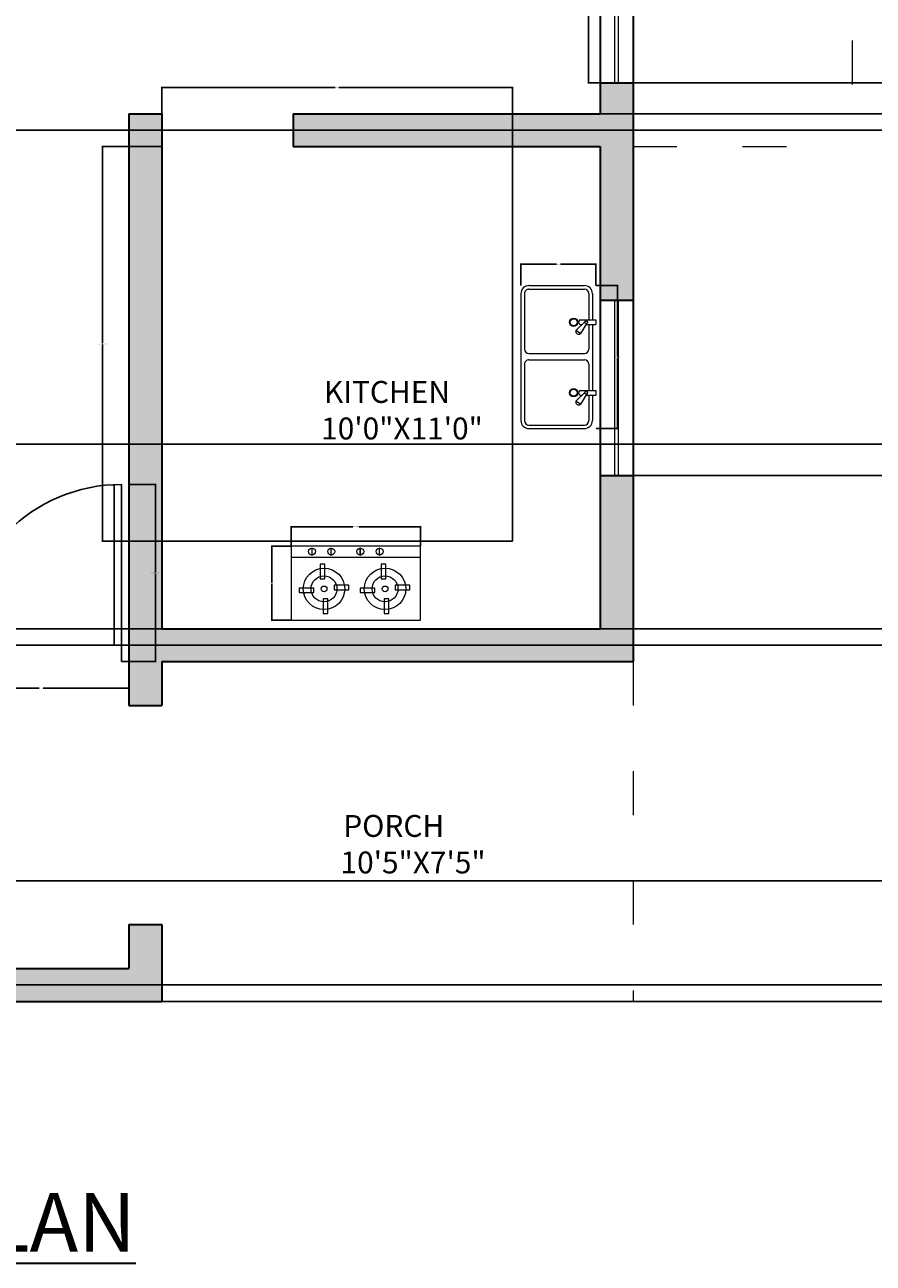
# Model space of a CAD drawing. Units: inches. Extents: x 5716 to 6907, y 12769 to 13594.
# Tile 2 of 17: x 6022 to 6254, y 12769 to 13109. Entities that reach past the tile are written whole.
import ezdxf

# ---------------------------------------------------------------- set-up
doc = ezdxf.new("R2010")
doc.units = ezdxf.units.IN
doc.linetypes.add('ACAD_ISO03W100', pattern=[30, 12, -18])
for name, color, linetype, lineweight in [('A-ANNO-DIMS', 2, 'Continuous', 18), ('A-ANNO-TEXT', 7, 'Continuous', 30), ('A-AREA-IDEN', 7, 'Continuous', 18), ('A-DOOR', 4, 'Continuous', 25), ('A-EQPM', 8, 'Continuous', 18), ('A-FLOR-CASE', 7, 'Continuous', 25), ('A-FLOR-FIXT', 9, 'Continuous', 18), ('A-FLOR-OVHD', 8, 'ACAD_ISO03W100', 18), ('A-GLAZ', 4, 'Continuous', 18), ('A-WALL', 7, 'Continuous', 35), ('A-WALL-PATT', 252, 'Continuous', 13)]:
    doc.layers.add(name, color=color, linetype=linetype, lineweight=lineweight)
doc.styles.get("Standard").update_dxf_attribs({"font": 'arial.ttf'})
doc.dimstyles.get("Standard").update_dxf_attribs({"dimtxt": 0.18, "dimasz": 0.18, "dimexe": 0.18, "dimexo": 0.0625, "dimgap": 0.09, "dimtad": 0, "dimtih": 1, "dimtoh": 1, "dimdec": 4, "dimzin": 0, "dimdsep": 46, "dimtxsty": 'Standard', "dimcen": 0.09, "dimadec": 0, "dimazin": 0, "dimtfac": 1, "dimtdec": 4, "dimtofl": 0, "dimtmove": 0, "dimatfit": 3, "dimfxl": 1, "dimtolj": 1, "dimtzin": 0, "dimarcsym": 0})

# ---------------------------------------------------------------- blocks, each defined once
blk = doc.blocks.new('A$C233D5AEA')
at = {"ltscale": 1000}
for p, q in [((375, 800), (65, 800)), ((375, 780), (65, 780)), ((20, 613.1), (20, 755)), ((40, 613.1), (40, 755)), ((400, 440), (400, 755)), ((420, 45), (420, 755)), ((51.1, 606.3), (87.4, 663.6)), ((111.9, 647), (62.8, 597.6)), ((87.4, 663.6), (111.9, 647)), ((55.4, 613.1), (0, 613.1)), ((0, 586.1), (0, 613.1)), ((88.6, 586.1), (0, 586.1)), ((20, 217.6), (20, 586.1)), ((40, 440), (40, 586.1)), ((87.8, 613.1), (78.2, 613.1)), ((40, 217.6), (40, 355)), ((375, 415), (65, 415)), ((375, 380), (65, 380)), ((400, 45), (400, 355)), ((55.4, 217.6), (0, 217.6)), ((0, 190.6), (0, 217.6)), ((51.1, 210.7), (87.4, 268)), ((111.9, 251.5), (62.8, 202)), ((87.8, 217.6), (78.2, 217.6)), ((87.4, 268), (111.9, 251.5)), ((88.6, 190.6), (0, 190.6)), ((20, 45), (20, 190.6)), ((40, 45), (40, 190.6)), ((375, 20), (65, 20)), ((375, 0), (65, 0))]:
    blk.add_line(p, q, dxfattribs=at)
for centre, radius in [((55.3, 599.7), 7.79), ((124.6, 599.4), 23.1), ((124.5, 599.4), 19.5), ((55.3, 204.2), 7.79), ((124.6, 204.7), 23.1), ((124.5, 204.7), 19.5)]:
    blk.add_circle(centre, radius, dxfattribs=at)
for centre, radius, start, end in [((65, 755), 45, 90, 180), ((65, 755), 25, 90, 180), ((375, 755), 45, 0, 90), ((375, 755), 25, 0, 90), ((97.5, 652.1), 15.3, 340.46224, 131.65496), ((82, 599.4), 14.9, 296.62368, 67.07956), ((65, 440), 25, 180, 270), ((375, 440), 25, 270, 0), ((65, 355), 25, 90, 180), ((375, 355), 25, 0, 90), ((97.5, 256.6), 15.3, 340.46913, 131.64807), ((82, 203.8), 14.9, 296.62368, 67.07956), ((65, 45), 45, 180, 270), ((65, 45), 25, 180, 270), ((375, 45), 45, 270, 0), ((375, 45), 25, 270, 0)]:
    blk.add_arc(centre, radius, start, end, dxfattribs=at)
blk = doc.blocks.new('A$C3BE07067')
at = {"rotation": 270}
blk.add_blockref('A$C233D5AEA', (0, 420), dxfattribs=at)
blk = doc.blocks.new('A$C67D72025')
at = {"ltscale": 1000}
for p, q in [((385.7, 234.1), (385.7, 209.4)), ((464.6, 234.1), (385.7, 234.1)), ((385.7, 209.4), (464.6, 209.4)), ((464.6, 209.4), (464.6, 234.1)), ((694.4, 59.5), (0, 59.5))]:
    blk.add_line(p, q, dxfattribs=at)
for points in [[(694.4, 396.8), (0, 396.8), (0, 0), (694.4, 0)], [(195.5, 283.6), (195.5, 362.4), (170.8, 362.4), (170.8, 283.6)], [(523.4, 283.6), (523.4, 362.4), (498.6, 362.4), (498.6, 283.6)], [(136.8, 234.1), (57.9, 234.1), (57.9, 209.4), (136.8, 209.4)], [(245, 224.8), (323.9, 224.8), (323.9, 249.5), (245, 249.5)], [(572.8, 224.8), (651.7, 224.8), (651.7, 249.5), (572.8, 249.5)], [(186.3, 175.3), (186.3, 96.5), (211, 96.5), (211, 175.3)], [(514.1, 175.3), (514.1, 96.5), (538.8, 96.5), (538.8, 175.3)], [(223.3, 47.3), (220, 47.3), (220, 9.9), (223.3, 9.9)], [(325.5, 47.3), (322.2, 47.3), (322.2, 9.9), (325.5, 9.9)], [(482.8, 47.3), (479.5, 47.3), (479.5, 9.9), (482.8, 9.9)], [(585, 47.3), (581.6, 47.3), (581.6, 9.9), (585, 9.9)]]:
    blk.add_lwpolyline(points, close=True, dxfattribs=at)
for centre, radius in [((190.9, 229.4), 111.3), ((518.7, 229.4), 111.3), ((190.9, 229.4), 69.6), ((518.7, 229.4), 69.6), ((190.9, 229.4), 15.5), ((518.7, 229.4), 15.5), ((220.3, 28.6), 18.6), ((323.9, 28.6), 18.6), ((480.1, 28.6), 18.6), ((583.7, 28.6), 18.6)]:
    blk.add_circle(centre, radius, dxfattribs=at)
blk = doc.blocks.new('DOOR-SWING-48IN')
for p, q in [((-2, 43.95), (-2, 0)), ((0, 44), (0, 0)), ((-46, 0), (-44, 0)), ((-44, 0), (-44, -4.5)), ((0, 0), (-2, 0)), ((2, 0), (0, 0)), ((0, 0), (0, -4.5)), ((-44, -4.5), (-46, -4.5)), ((0, -4.5), (2, -4.5))]:
    blk.add_line(p, q)
blk.add_arc((0, 0), 44, 90, 180)
blk = doc.blocks.new('WIN-GLAZING-48IN')
for p, q in [((0, 0), (0, 48)), ((1, 0), (1, 48))]:
    blk.add_line(p, q)
blk = doc.blocks.new('COUNTER-L-KITCHEN')
for p in [(0, 108), (-96, 0)]:
    blk.add_line(p, (0, 0))
blk = doc.blocks.new('*D31')
at = {"layer": 'A-ANNO-DIMS', "color": 0, "lineweight": -2, "transparency": 16777216}
for p, q in [((6182.96, 13140.65), (6175.64, 13140.65)), ((6175.82, 13140.47), (6175.82, 13116.83)), ((6175.82, 13092.83), (6175.82, 13116.47)), ((6182.96, 13092.65), (6175.64, 13092.65))]:
    blk.add_line(p, q, dxfattribs=at)
at = {"layer": 'A-ANNO-DIMS', "color": 0, "transparency": 16777216}
for points in [[(6175.79, 13140.47), (6175.85, 13140.47), (6175.82, 13140.65)], [(6175.79, 13092.83), (6175.85, 13092.83), (6175.82, 13092.65)]]:
    blk.add_solid(points, dxfattribs=at)
at = {"layer": 'Defpoints', "color": 0, "transparency": 16777216}
for p in [(6175.82, 13140.65), (6183.02, 13140.65), (6183.02, 13092.65)]:
    blk.add_point(p, dxfattribs=at)
at = {"layer": 'A-ANNO-DIMS', "color": 0, "transparency": 16777216, "insert": (6175.82, 13116.65), "char_height": 0.18, "attachment_point": 5}
blk.add_mtext('\\A1;WINDOW 48 TYP.', dxfattribs=at)
blk = doc.blocks.new('*D35')
at = {"layer": 'A-ANNO-DIMS', "color": 0, "lineweight": -2, "transparency": 16777216}
for p, q in [((6177.95, 13037.09), (6183.94, 13037.09)), ((6183.76, 13036.91), (6183.76, 13017.7)), ((6183.76, 12998.12), (6183.76, 13017.33)), ((6177.95, 12997.94), (6183.94, 12997.94))]:
    blk.add_line(p, q, dxfattribs=at)
at = {"layer": 'A-ANNO-DIMS', "color": 0, "transparency": 16777216}
for points in [[(6183.73, 13036.91), (6183.79, 13036.91), (6183.76, 13037.09)], [(6183.73, 12998.12), (6183.79, 12998.12), (6183.76, 12997.94)]]:
    blk.add_solid(points, dxfattribs=at)
at = {"layer": 'Defpoints', "color": 0, "transparency": 16777216}
for p in [(6177.88, 13037.09), (6177.88, 12997.94), (6183.76, 12997.94)]:
    blk.add_point(p, dxfattribs=at)
at = {"layer": 'A-ANNO-DIMS', "color": 0, "transparency": 16777216, "insert": (6183.76, 13017.51), "char_height": 0.18, "attachment_point": 5}
blk.add_mtext('\\A1;SINK 39 TYP.', dxfattribs=at)
blk = doc.blocks.new('*D36')
at = {"layer": 'A-ANNO-DIMS', "color": 0, "lineweight": -2, "transparency": 16777216}
for p, q in [((6157.33, 13037.15), (6157.33, 13043.14)), ((6157.51, 13042.96), (6167.08, 13042.96)), ((6177.7, 13042.96), (6168.14, 13042.96)), ((6177.88, 13037.15), (6177.88, 13043.14))]:
    blk.add_line(p, q, dxfattribs=at)
at = {"layer": 'A-ANNO-DIMS', "color": 0, "transparency": 16777216}
for points in [[(6157.51, 13042.99), (6157.51, 13042.93), (6157.33, 13042.96)], [(6177.7, 13042.99), (6177.7, 13042.93), (6177.88, 13042.96)]]:
    blk.add_solid(points, dxfattribs=at)
at = {"layer": 'Defpoints', "color": 0, "transparency": 16777216}
for p in [(6177.88, 13042.96), (6157.33, 13037.09), (6177.88, 13037.09)]:
    blk.add_point(p, dxfattribs=at)
at = {"layer": 'A-ANNO-DIMS', "color": 0, "transparency": 16777216, "insert": (6167.61, 13042.96), "char_height": 0.18, "attachment_point": 5}
blk.add_mtext('\\A1;21 TYP.', dxfattribs=at)
blk = doc.blocks.new('*D39')
at = {"layer": 'A-ANNO-DIMS', "color": 0, "lineweight": -2, "transparency": 16777216}
for p, q in [((6094.5, 12965.82), (6094.5, 12971.24)), ((6094.68, 12971.06), (6111.36, 12971.06)), ((6129.7, 12971.06), (6113.02, 12971.06)), ((6129.88, 12965.82), (6129.88, 12971.24))]:
    blk.add_line(p, q, dxfattribs=at)
at = {"layer": 'A-ANNO-DIMS', "color": 0, "transparency": 16777216}
for points in [[(6094.68, 12971.09), (6094.68, 12971.03), (6094.5, 12971.06)], [(6129.7, 12971.09), (6129.7, 12971.03), (6129.88, 12971.06)]]:
    blk.add_solid(points, dxfattribs=at)
at = {"layer": 'Defpoints', "color": 0, "transparency": 16777216}
for p in [(6094.5, 12971.06), (6094.5, 12965.75), (6129.88, 12965.75)]:
    blk.add_point(p, dxfattribs=at)
at = {"layer": 'A-ANNO-DIMS', "color": 0, "transparency": 16777216, "insert": (6112.19, 12971.06), "char_height": 0.18, "attachment_point": 5}
blk.add_mtext('\\A1;HOB 35 TYP.', dxfattribs=at)
blk = doc.blocks.new('*D40')
at = {"layer": 'A-ANNO-DIMS', "color": 0, "lineweight": -2, "transparency": 16777216}
for p, q in [((6094.44, 12965.75), (6089.02, 12965.75)), ((6089.2, 12965.57), (6089.2, 12955.83)), ((6089.2, 12945.72), (6089.2, 12955.46)), ((6094.44, 12945.54), (6089.02, 12945.54))]:
    blk.add_line(p, q, dxfattribs=at)
at = {"layer": 'A-ANNO-DIMS', "color": 0, "transparency": 16777216}
for points in [[(6089.17, 12965.57), (6089.23, 12965.57), (6089.2, 12965.75)], [(6089.17, 12945.72), (6089.23, 12945.72), (6089.2, 12945.54)]]:
    blk.add_solid(points, dxfattribs=at)
at = {"layer": 'Defpoints', "color": 0, "transparency": 16777216}
for p in [(6094.5, 12965.75), (6089.2, 12945.54), (6094.5, 12945.54)]:
    blk.add_point(p, dxfattribs=at)
at = {"layer": 'A-ANNO-DIMS', "color": 0, "transparency": 16777216, "insert": (6089.2, 12955.64), "char_height": 0.18, "attachment_point": 5}
blk.add_mtext('\\A1;20 TYP.', dxfattribs=at)
blk = doc.blocks.new('*D41')
at = {"layer": 'A-ANNO-DIMS', "color": 0, "lineweight": -2, "transparency": 16777216}
for p, q in [((6050.09, 12982.65), (6057.48, 12982.65)), ((6057.3, 12982.47), (6057.3, 12958.58)), ((6057.3, 12934.33), (6057.3, 12958.22)), ((6050.09, 12934.15), (6057.48, 12934.15))]:
    blk.add_line(p, q, dxfattribs=at)
at = {"layer": 'A-ANNO-DIMS', "color": 0, "transparency": 16777216}
for points in [[(6057.27, 12982.47), (6057.33, 12982.47), (6057.3, 12982.65)], [(6057.27, 12934.33), (6057.33, 12934.33), (6057.3, 12934.15)]]:
    blk.add_solid(points, dxfattribs=at)
at = {"layer": 'Defpoints', "color": 0, "transparency": 16777216}
for p in [(6050.02, 12982.65), (6057.3, 12982.65), (6050.02, 12934.15)]:
    blk.add_point(p, dxfattribs=at)
at = {"layer": 'A-ANNO-DIMS', "color": 0, "transparency": 16777216, "insert": (6057.3, 12958.4), "char_height": 0.18, "attachment_point": 5}
blk.add_mtext('\\A1;ENTRY DOOR 49 TYP.', dxfattribs=at)
blk = doc.blocks.new('*D42')
at = {"layer": 'A-ANNO-DIMS', "color": 0, "lineweight": -2, "transparency": 16777216}
for p, q in [((6002.02, 12934.09), (6002.02, 12926.69)), ((6050.02, 12934.09), (6050.02, 12926.69)), ((6002.2, 12926.87), (6025.49, 12926.87)), ((6049.84, 12926.87), (6026.55, 12926.87))]:
    blk.add_line(p, q, dxfattribs=at)
at = {"layer": 'A-ANNO-DIMS', "color": 0, "transparency": 16777216}
for points in [[(6002.2, 12926.9), (6002.2, 12926.84), (6002.02, 12926.87)], [(6049.84, 12926.9), (6049.84, 12926.84), (6050.02, 12926.87)]]:
    blk.add_solid(points, dxfattribs=at)
at = {"layer": 'Defpoints', "color": 0, "transparency": 16777216}
for p in [(6002.02, 12934.15), (6050.02, 12934.15), (6050.02, 12926.87)]:
    blk.add_point(p, dxfattribs=at)
at = {"layer": 'A-ANNO-DIMS', "color": 0, "transparency": 16777216, "insert": (6026.02, 12926.87), "char_height": 0.18, "attachment_point": 5}
blk.add_mtext('\\A1;48 TYP.', dxfattribs=at)
blk = doc.blocks.new('*D47')
at = {"layer": 'A-ANNO-DIMS', "color": 0, "lineweight": -2, "transparency": 16777216}
for p, q in [((6058.96, 13075.15), (6042.64, 13075.15)), ((6042.82, 13074.97), (6042.82, 13021.33)), ((6042.82, 12967.33), (6042.82, 13020.97)), ((6058.96, 12967.15), (6042.64, 12967.15))]:
    blk.add_line(p, q, dxfattribs=at)
at = {"layer": 'A-ANNO-DIMS', "color": 0, "transparency": 16777216}
for points in [[(6042.79, 13074.97), (6042.85, 13074.97), (6042.82, 13075.15)], [(6042.79, 12967.33), (6042.85, 12967.33), (6042.82, 12967.15)]]:
    blk.add_solid(points, dxfattribs=at)
at = {"layer": 'Defpoints', "color": 0, "transparency": 16777216}
for p in [(6042.82, 13075.15), (6059.02, 13075.15), (6059.02, 12967.15)]:
    blk.add_point(p, dxfattribs=at)
at = {"layer": 'A-ANNO-DIMS', "color": 0, "transparency": 16777216, "insert": (6042.82, 13021.15), "char_height": 0.18, "attachment_point": 5}
blk.add_mtext('\\A1;L-COUNTER 108 TYP.', dxfattribs=at)
blk = doc.blocks.new('*D48')
at = {"layer": 'A-ANNO-DIMS', "color": 0, "lineweight": -2, "transparency": 16777216}
for p, q in [((6059.02, 13075.21), (6059.02, 13091.53)), ((6059.2, 13091.35), (6106.49, 13091.35)), ((6154.84, 13091.35), (6107.55, 13091.35)), ((6155.02, 13075.21), (6155.02, 13091.53))]:
    blk.add_line(p, q, dxfattribs=at)
at = {"layer": 'A-ANNO-DIMS', "color": 0, "transparency": 16777216}
for points in [[(6059.2, 13091.38), (6059.2, 13091.32), (6059.02, 13091.35)], [(6154.84, 13091.38), (6154.84, 13091.32), (6155.02, 13091.35)]]:
    blk.add_solid(points, dxfattribs=at)
at = {"layer": 'Defpoints', "color": 0, "transparency": 16777216}
for p in [(6155.02, 13091.35), (6059.02, 13075.15), (6155.02, 13075.15)]:
    blk.add_point(p, dxfattribs=at)
at = {"layer": 'A-ANNO-DIMS', "color": 0, "transparency": 16777216, "insert": (6107.02, 13091.35), "char_height": 0.18, "attachment_point": 5}
blk.add_mtext('\\A1;96 TYP.', dxfattribs=at)
blk = doc.blocks.new('*D52')
at = {"layer": 'A-ANNO-DIMS', "color": 0, "lineweight": -2, "transparency": 16777216}
for p, q in [((6267.34, 13440.15), (5716.04, 13440.15)), ((5716.22, 13439.97), (5716.22, 13140.83)), ((5716.22, 12841.33), (5716.22, 13140.47)), ((6267.34, 12841.15), (5716.04, 12841.15))]:
    blk.add_line(p, q, dxfattribs=at)
at = {"layer": 'A-ANNO-DIMS', "color": 0, "transparency": 16777216}
for points in [[(5716.19, 13439.97), (5716.25, 13439.97), (5716.22, 13440.15)], [(5716.19, 12841.33), (5716.25, 12841.33), (5716.22, 12841.15)]]:
    blk.add_solid(points, dxfattribs=at)
at = {"layer": 'Defpoints', "color": 0, "transparency": 16777216}
for p in [(6267.41, 13440.15), (5716.22, 12841.15), (6267.41, 12841.15)]:
    blk.add_point(p, dxfattribs=at)
at = {"layer": 'A-ANNO-DIMS', "color": 0, "transparency": 16777216, "insert": (5716.22, 13140.65), "char_height": 0.18, "attachment_point": 5}
blk.add_mtext('\\A1;599', dxfattribs=at)
blk = doc.blocks.new('*D62')
at = {"layer": 'A-ANNO-DIMS', "color": 0, "lineweight": -2, "transparency": 16777216}
for p, q in [((6736.67, 13120.65), (5716.04, 13120.65)), ((5716.22, 13120.47), (5716.22, 13100.33)), ((5716.22, 13079.83), (5716.22, 13099.97)), ((6736.67, 13079.65), (5716.04, 13079.65))]:
    blk.add_line(p, q, dxfattribs=at)
at = {"layer": 'A-ANNO-DIMS', "color": 0, "transparency": 16777216}
for points in [[(5716.19, 13120.47), (5716.25, 13120.47), (5716.22, 13120.65)], [(5716.19, 13079.83), (5716.25, 13079.83), (5716.22, 13079.65)]]:
    blk.add_solid(points, dxfattribs=at)
at = {"layer": 'Defpoints', "color": 0, "transparency": 16777216}
for p in [(6736.73, 13120.65), (5716.22, 13079.65), (6736.73, 13079.65)]:
    blk.add_point(p, dxfattribs=at)
at = {"layer": 'A-ANNO-DIMS', "color": 0, "transparency": 16777216, "insert": (5716.22, 13100.15), "char_height": 0.18, "attachment_point": 5}
blk.add_mtext('\\A1;41', dxfattribs=at)
blk = doc.blocks.new('*D63')
at = {"layer": 'A-ANNO-DIMS', "color": 0, "lineweight": -2, "transparency": 16777216}
for p, q in [((6736.67, 13079.65), (5716.04, 13079.65)), ((5716.22, 13079.47), (5716.22, 13009.33)), ((5716.22, 12938.83), (5716.22, 13008.97)), ((6736.67, 12938.65), (5716.04, 12938.65))]:
    blk.add_line(p, q, dxfattribs=at)
at = {"layer": 'A-ANNO-DIMS', "color": 0, "transparency": 16777216}
for points in [[(5716.19, 13079.47), (5716.25, 13079.47), (5716.22, 13079.65)], [(5716.19, 12938.83), (5716.25, 12938.83), (5716.22, 12938.65)]]:
    blk.add_solid(points, dxfattribs=at)
at = {"layer": 'Defpoints', "color": 0, "transparency": 16777216}
for p in [(6736.73, 13079.65), (5716.22, 12938.65), (6736.73, 12938.65)]:
    blk.add_point(p, dxfattribs=at)
at = {"layer": 'A-ANNO-DIMS', "color": 0, "transparency": 16777216, "insert": (5716.22, 13009.15), "char_height": 0.18, "attachment_point": 5}
blk.add_mtext('\\A1;141', dxfattribs=at)
blk = doc.blocks.new('*D64')
at = {"layer": 'A-ANNO-DIMS', "color": 0, "lineweight": -2, "transparency": 16777216}
for p, q in [((6736.67, 12938.65), (5716.04, 12938.65)), ((5716.22, 12938.47), (5716.22, 12892.33)), ((5716.22, 12845.83), (5716.22, 12891.97)), ((6736.67, 12845.65), (5716.04, 12845.65))]:
    blk.add_line(p, q, dxfattribs=at)
at = {"layer": 'A-ANNO-DIMS', "color": 0, "transparency": 16777216}
for points in [[(5716.19, 12938.47), (5716.25, 12938.47), (5716.22, 12938.65)], [(5716.19, 12845.83), (5716.25, 12845.83), (5716.22, 12845.65)]]:
    blk.add_solid(points, dxfattribs=at)
at = {"layer": 'Defpoints', "color": 0, "transparency": 16777216}
for p in [(6736.73, 12938.65), (5716.22, 12845.65), (6736.73, 12845.65)]:
    blk.add_point(p, dxfattribs=at)
at = {"layer": 'A-ANNO-DIMS', "color": 0, "transparency": 16777216, "insert": (5716.22, 12892.15), "char_height": 0.18, "attachment_point": 5}
blk.add_mtext('\\A1;93', dxfattribs=at)
blk = doc.blocks.new('*D67')
at = {"layer": 'A-ANNO-DIMS', "color": 0, "lineweight": -2, "transparency": 16777216}
for p, q in [((5819.09, 12874.15), (6907.26, 12874.15)), ((6907.08, 12873.97), (6907.08, 12857.83)), ((6907.08, 12841.33), (6907.08, 12857.47)), ((5819.09, 12841.15), (6907.26, 12841.15))]:
    blk.add_line(p, q, dxfattribs=at)
at = {"layer": 'A-ANNO-DIMS', "color": 0, "transparency": 16777216}
for points in [[(6907.05, 12873.97), (6907.11, 12873.97), (6907.08, 12874.15)], [(6907.05, 12841.33), (6907.11, 12841.33), (6907.08, 12841.15)]]:
    blk.add_solid(points, dxfattribs=at)
at = {"layer": 'Defpoints', "color": 0, "transparency": 16777216}
for p in [(5819.02, 12874.15), (6907.08, 12874.15), (5819.02, 12841.15)]:
    blk.add_point(p, dxfattribs=at)
at = {"layer": 'A-ANNO-DIMS', "color": 0, "transparency": 16777216, "insert": (6907.08, 12857.65), "char_height": 0.18, "attachment_point": 5}
blk.add_mtext('\\A1;33', dxfattribs=at)
blk = doc.blocks.new('*D68')
at = {"layer": 'A-ANNO-DIMS', "color": 0, "lineweight": -2, "transparency": 16777216}
for p, q in [((5828.09, 12993.65), (6907.26, 12993.65)), ((6907.08, 12993.47), (6907.08, 12968.58)), ((6907.08, 12943.33), (6907.08, 12968.22)), ((5828.09, 12943.15), (6907.26, 12943.15))]:
    blk.add_line(p, q, dxfattribs=at)
at = {"layer": 'A-ANNO-DIMS', "color": 0, "transparency": 16777216}
for points in [[(6907.05, 12993.47), (6907.11, 12993.47), (6907.08, 12993.65)], [(6907.05, 12943.33), (6907.11, 12943.33), (6907.08, 12943.15)]]:
    blk.add_solid(points, dxfattribs=at)
at = {"layer": 'Defpoints', "color": 0, "transparency": 16777216}
for p in [(5828.02, 12993.65), (6907.08, 12993.65), (5828.02, 12943.15)]:
    blk.add_point(p, dxfattribs=at)
at = {"layer": 'A-ANNO-DIMS', "color": 0, "transparency": 16777216, "insert": (6907.08, 12968.4), "char_height": 0.18, "attachment_point": 5}
blk.add_mtext('\\A1;50.5', dxfattribs=at)
blk = doc.blocks.new('*D72')
at = {"layer": 'A-ANNO-DIMS', "color": 0, "lineweight": -2, "transparency": 16777216}
for p, q in [((6188.09, 12985.15), (6907.26, 12985.15)), ((6907.08, 12984.97), (6907.08, 12964.33)), ((6907.08, 12943.33), (6907.08, 12963.97)), ((6179.09, 12943.15), (6907.26, 12943.15))]:
    blk.add_line(p, q, dxfattribs=at)
at = {"layer": 'A-ANNO-DIMS', "color": 0, "transparency": 16777216}
for points in [[(6907.05, 12984.97), (6907.11, 12984.97), (6907.08, 12985.15)], [(6907.05, 12943.33), (6907.11, 12943.33), (6907.08, 12943.15)]]:
    blk.add_solid(points, dxfattribs=at)
at = {"layer": 'Defpoints', "color": 0, "transparency": 16777216}
for p in [(6188.02, 12985.15), (6907.08, 12985.15), (6179.02, 12943.15)]:
    blk.add_point(p, dxfattribs=at)
at = {"layer": 'A-ANNO-DIMS', "color": 0, "transparency": 16777216, "insert": (6907.08, 12964.15), "char_height": 0.18, "attachment_point": 5}
blk.add_mtext('\\A1;42', dxfattribs=at)
blk = doc.blocks.new('*D73')
at = {"layer": 'A-ANNO-DIMS', "color": 0, "lineweight": -2, "transparency": 16777216}
for p, q in [((6188.09, 13092.65), (6907.26, 13092.65)), ((6907.08, 13092.47), (6907.08, 13088.58)), ((6907.08, 13084.33), (6907.08, 13088.22)), ((6179.09, 13084.15), (6907.26, 13084.15))]:
    blk.add_line(p, q, dxfattribs=at)
at = {"layer": 'A-ANNO-DIMS', "color": 0, "transparency": 16777216}
for points in [[(6907.05, 13092.47), (6907.11, 13092.47), (6907.08, 13092.65)], [(6907.05, 13084.33), (6907.11, 13084.33), (6907.08, 13084.15)]]:
    blk.add_solid(points, dxfattribs=at)
at = {"layer": 'Defpoints', "color": 0, "transparency": 16777216}
for p in [(6188.02, 13092.65), (6907.08, 13092.65), (6179.02, 13084.15)]:
    blk.add_point(p, dxfattribs=at)
at = {"layer": 'A-ANNO-DIMS', "color": 0, "transparency": 16777216, "insert": (6907.08, 13088.4), "char_height": 0.18, "attachment_point": 5}
blk.add_mtext('\\A1;8.5', dxfattribs=at)

msp = doc.modelspace()

# ---------------------------------------------------------------- hatches: boundary and pattern name
at = {"layer": 'A-WALL-PATT'}
h = msp.add_hatch(color=256, dxfattribs=at)
h.dxf.hatch_style = 1
h.paths.add_polyline_path([(6188.02, 13092.65), (6179.02, 13092.65), (6179.02, 13084.15), (6095.02, 13084.15), (6095.02, 13075.15), (6179.02, 13075.15), (6179.02, 13033.15), (6188.02, 13033.15)])
h = msp.add_hatch(color=256, dxfattribs=at)
h.dxf.hatch_style = 1
h.paths.add_polyline_path([(6059.02, 13084.15), (6050.02, 13084.15), (6050.02, 12922.15), (6059.02, 12922.15), (6059.02, 12934.15), (6188.02, 12934.15), (6188.02, 12985.15), (6179.02, 12985.15), (6179.02, 12943.15), (6059.02, 12943.15)])
h = msp.add_hatch(color=256, dxfattribs=at)
h.dxf.hatch_style = 1
h.paths.add_polyline_path([(6059.02, 12862.15), (6050.02, 12862.15), (6050.02, 12850.15), (5828.02, 12850.15), (5828.02, 12874.15), (5819.02, 12874.15), (5819.02, 12841.15), (6059.02, 12841.15)])

# ---------------------------------------------------------------- linework, layer by layer
at = {"layer": 'A-FLOR-OVHD'}
for p, q in [((6248.02, 13194.15), (6248.02, 13075.15)), ((6188.02, 13075.15), (6248.02, 13075.15)), ((6188.02, 12934.15), (6188.02, 12841.15)), ((6059.02, 12841.15), (6188.02, 12841.15))]:
    msp.add_line(p, q, dxfattribs=at)
at = {"layer": 'A-WALL'}
for p, q in [((6179.02, 13149.15), (6179.02, 13084.15)), ((6188.02, 13149.15), (6188.02, 12934.15)), ((6179.02, 13092.65), (6188.02, 13092.65)), ((6050.02, 13084.15), (6059.02, 13084.15)), ((6050.02, 13084.15), (6050.02, 12922.15)), ((6059.02, 13084.15), (6059.02, 12943.15)), ((6095.02, 13084.15), (6095.02, 13075.15)), ((6095.02, 13084.15), (6179.02, 13084.15)), ((6095.02, 13075.15), (6179.02, 13075.15)), ((6179.02, 13075.15), (6179.02, 12943.15)), ((6179.02, 13033.15), (6188.02, 13033.15)), ((6179.02, 12985.15), (6188.02, 12985.15)), ((6059.02, 12943.15), (6179.02, 12943.15)), ((6059.02, 12934.15), (6188.02, 12934.15)), ((6059.02, 12934.15), (6059.02, 12922.15)), ((6050.02, 12922.15), (6059.02, 12922.15)), ((6050.02, 12862.15), (6059.02, 12862.15)), ((6050.02, 12862.15), (6050.02, 12850.15)), ((6059.02, 12862.15), (6059.02, 12841.15)), ((5828.02, 12850.15), (6050.02, 12850.15)), ((5819.02, 12841.15), (6059.02, 12841.15))]:
    msp.add_line(p, q, dxfattribs=at)

# ---------------------------------------------------------------- block references
at = {"layer": 'A-DOOR'}
msp.add_blockref('DOOR-SWING-48IN', (6048.02, 12938.65), dxfattribs=at)
at = {"layer": 'A-EQPM', "xscale": 0.0509457092912183, "yscale": 0.0509457092912183, "zscale": 0.0509457092912183, "rotation": 180}
msp.add_blockref('A$C67D72025', (6129.88, 12965.75), dxfattribs=at)
at = {"layer": 'A-FLOR-CASE'}
msp.add_blockref('COUNTER-L-KITCHEN', (6155.02, 12967.15), dxfattribs=at)
at = {"layer": 'A-FLOR-FIXT', "xscale": 0.0489344977334652, "yscale": 0.0489344977334652, "zscale": 0.0489344977334652, "rotation": 270}
msp.add_blockref('A$C3BE07067', (6157.33, 13037.09), dxfattribs=at)
at = {"layer": 'A-GLAZ'}
for p in [(6183.02, 13092.65), (6183.02, 12985.15)]:
    msp.add_blockref('WIN-GLAZING-48IN', p, dxfattribs=at)

# ---------------------------------------------------------------- texts
at = {"layer": 'A-ANNO-TEXT', "insert": (5922.18, 12788.65), "char_height": 16, "attachment_point": 1}
msp.add_mtext_dynamic_manual_height_columns('{\\LFLOOR PLAN}', width=852.8728, gutter_width=12.5, heights=[0], dxfattribs=at)
at = {"layer": 'A-AREA-IDEN', "char_height": 2.5, "attachment_point": 1}
for s, width, heights, insert in [(' {\\H2.4x;KITCHEN\\P10\'0"X11\'0"}', 81.2135, [0], (6102.66, 13010.98)), (' {\\H2.4x;PORCH\\P10\'5"X7\'5"}', 95.0073, [19.73], (6107.96, 12892.17))]:
    msp.add_mtext_dynamic_manual_height_columns(s, width=width, gutter_width=12.5, heights=heights, dxfattribs=dict(at, insert=insert))

# ---------------------------------------------------------------- dimensions: what is measured, and where the dimension line sits
at = {"layer": 'A-ANNO-DIMS'}
for base, p1, p2, override, picture, middle in [((5716.22, 12841.15), (6267.41, 13440.15), (6267.41, 12841.15), {"dimdec": 0, "dimlfac": 1, "dimrnd": 0, "dimzin": 0, "dimdsep": 46, "dimlunit": 2}, '*D52', (5716.22, 13140.65)), ((5716.22, 13079.65), (6736.73, 13120.65), (6736.73, 13079.65), {"dimdec": 0, "dimlfac": 1, "dimrnd": 0, "dimzin": 0, "dimdsep": 46, "dimlunit": 2}, '*D62', (5716.22, 13100.15)), ((6907.08, 13092.65), (6179.02, 13084.15), (6188.02, 13092.65), {"dimdec": 1, "dimlfac": 1, "dimrnd": 0, "dimzin": 0, "dimdsep": 46, "dimlunit": 2}, '*D73', (6907.08, 13088.4)), ((5716.22, 12938.65), (6736.73, 13079.65), (6736.73, 12938.65), {"dimdec": 0, "dimlfac": 1, "dimrnd": 0, "dimzin": 0, "dimdsep": 46, "dimlunit": 2}, '*D63', (5716.22, 13009.15)), ((6907.08, 12993.65), (5828.02, 12943.15), (5828.02, 12993.65), {"dimdec": 1, "dimlfac": 1, "dimrnd": 0, "dimzin": 0, "dimdsep": 46, "dimlunit": 2}, '*D68', (6907.08, 12968.4)), ((6907.08, 12985.15), (6179.02, 12943.15), (6188.02, 12985.15), {"dimdec": 0, "dimlfac": 1, "dimrnd": 0, "dimzin": 0, "dimdsep": 46, "dimlunit": 2}, '*D72', (6907.08, 12964.15)), ((5716.22, 12845.65), (6736.73, 12938.65), (6736.73, 12845.65), {"dimdec": 0, "dimlfac": 1, "dimrnd": 0, "dimzin": 0, "dimdsep": 46, "dimlunit": 2}, '*D64', (5716.22, 12892.15)), ((6907.08, 12874.15), (5819.02, 12841.15), (5819.02, 12874.15), {"dimdec": 0, "dimlfac": 1, "dimrnd": 0, "dimzin": 0, "dimdsep": 46, "dimlunit": 2}, '*D67', (6907.08, 12857.65))]:
    dim = msp.add_linear_dim(base=base, p1=p1, p2=p2, angle=90, dimstyle='Standard', override=override, dxfattribs=at)
    dim.commit()
    dim.dimension.update_dxf_attribs({"geometry": picture, "text_midpoint": middle})
for base, p1, p2, angle, text, picture, middle in [((6175.82, 13140.65), (6183.02, 13092.65), (6183.02, 13140.65), 90, 'WINDOW <> TYP.', '*D31', (6175.82, 13116.65)), ((6042.82, 13075.15), (6059.02, 12967.15), (6059.02, 13075.15), 90, 'L-COUNTER <> TYP.', '*D47', (6042.82, 13021.15)), ((6183.76, 12997.94), (6177.88, 13037.09), (6177.88, 12997.94), 270, 'SINK <> TYP.', '*D35', (6183.76, 13017.51)), ((6057.29751723, 12982.64894948), (6050.02251723, 12934.14894948), (6050.02251723, 12982.64894948), 90, 'ENTRY DOOR <> TYP.', '*D41', (6057.29751723, 12958.39894948)), ((6094.5, 12971.06), (6129.88, 12965.75), (6094.5, 12965.75), 180, 'HOB <> TYP.', '*D39', (6112.19, 12971.06)), ((6089.2, 12945.54), (6094.5, 12965.75), (6094.5, 12945.54), 270, '<> TYP.', '*D40', (6089.2, 12955.64))]:
    dim = msp.add_linear_dim(base=base, p1=p1, p2=p2, angle=angle, text=text, dimstyle='Standard', override={"dimdec": 0, "dimlfac": 1, "dimrnd": 0, "dimzin": 0, "dimdsep": 46, "dimlunit": 2}, dxfattribs=at)
    dim.commit()
    dim.dimension.update_dxf_attribs({"geometry": picture, "text_midpoint": middle})
for base, p1, p2, picture, middle in [((6155.02, 13091.35), (6059.02, 13075.15), (6155.02, 13075.15), '*D48', (6107.02, 13091.35)), ((6177.88, 13042.96), (6157.33, 13037.09), (6177.88, 13037.09), '*D36', (6167.61, 13042.96)), ((6050.02, 12926.87), (6002.02, 12934.15), (6050.02, 12934.15), '*D42', (6026.02, 12926.87))]:
    dim = msp.add_linear_dim(base=base, p1=p1, p2=p2, text='<> TYP.', dimstyle='Standard', override={"dimdec": 0, "dimlfac": 1, "dimrnd": 0, "dimzin": 0, "dimdsep": 46, "dimlunit": 2}, dxfattribs=at)
    dim.commit()
    dim.dimension.update_dxf_attribs({"geometry": picture, "text_midpoint": middle})

doc.saveas('drawing.dxf')
